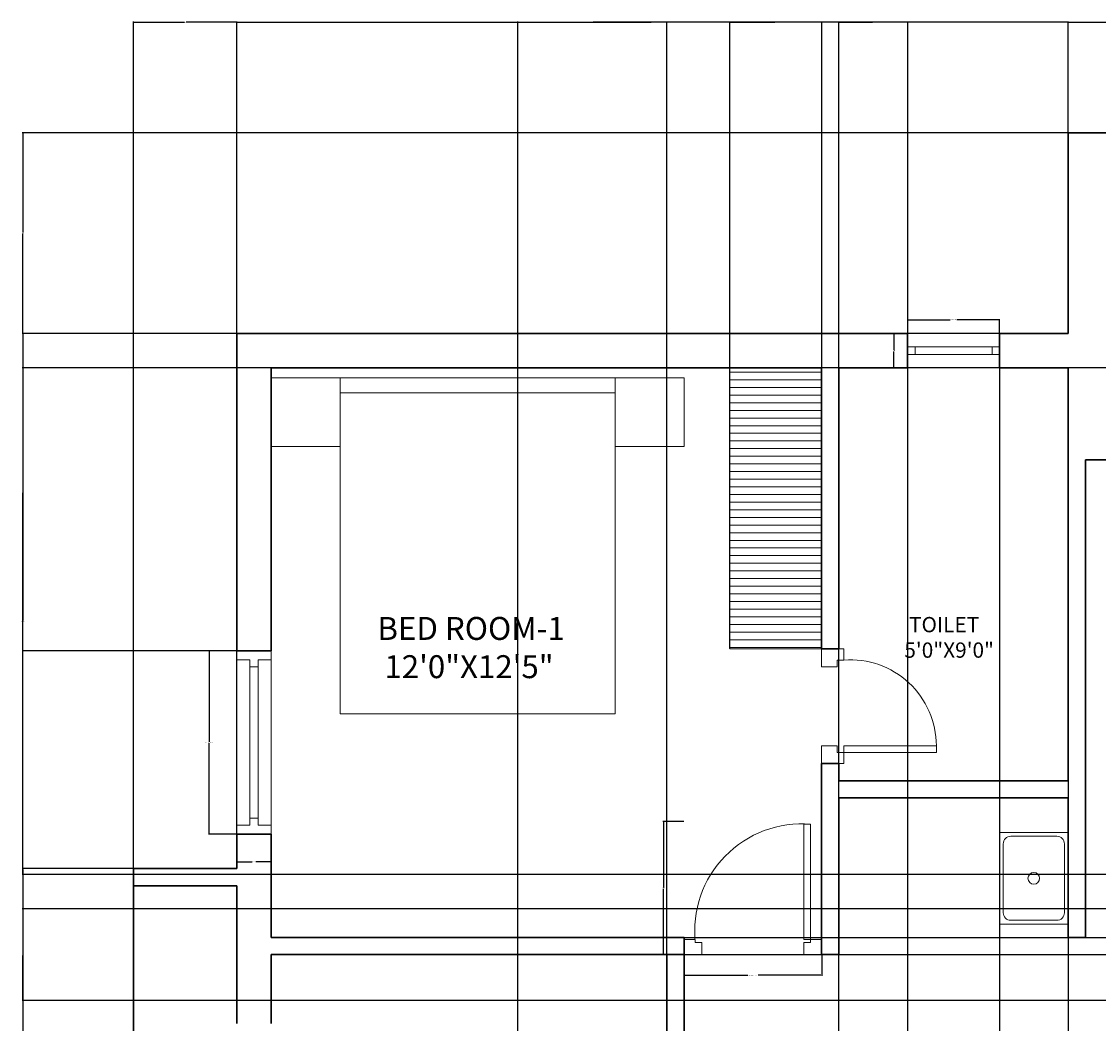
# Model space of a CAD drawing. Units: inches. Extents: x 2134 to 2768, y 715 to 1206.
# Tile 2 of 4: x 2134 to 2416, y 944 to 1206. Entities that reach past the tile are written whole.
import ezdxf

# ---------------------------------------------------------------- set-up
doc = ezdxf.new("R2010")
doc.units = ezdxf.units.IN
for name, color, linetype, lineweight in [('A-ANNO-DIMS', 2, 'Continuous', 18), ('A-AREA-IDEN', 7, 'Continuous', 18), ('A-DOOR', 251, 'Continuous', 13), ('A-FLOR-CASE', 251, 'Continuous', 13), ('A-FLOR-CASE-PATT', 252, 'Continuous', 9), ('A-FLOR-FIXT', 9, 'Continuous', 13), ('A-FURN', 251, 'Continuous', 13), ('A-WALL', 7, 'Continuous', 30), ('A-WINDOW', 251, 'Continuous', 13)]:
    doc.layers.add(name, color=color, linetype=linetype, lineweight=lineweight)
doc.styles.get("Standard").update_dxf_attribs({"font": 'arial.ttf'})
doc.dimstyles.get("Standard").update_dxf_attribs({"dimtxt": 0.18, "dimasz": 0.18, "dimexe": 0.18, "dimexo": 0.0625, "dimgap": 0.09, "dimtad": 0, "dimtih": 1, "dimtoh": 1, "dimdec": 4, "dimzin": 0, "dimdsep": 46, "dimtxsty": 'Standard', "dimcen": 0.09, "dimadec": 0, "dimazin": 0, "dimtfac": 1, "dimtdec": 4, "dimtofl": 0, "dimtmove": 0, "dimatfit": 3, "dimfxl": 1, "dimtolj": 1, "dimtzin": 0, "dimarcsym": 0})

# ---------------------------------------------------------------- blocks, each defined once
blk = doc.blocks.new('ARCHITRAVE')
at = {"layer": 'A-DOOR'}
for p, q in [((0, 0), (0, 4)), ((0, 3.99), (2.92, 3.99)), ((2.92, 3.99), (2.92, 3.17)), ((2.92, 3.17), (4.67, 3.17)), ((4.67, 3.17), (4.67, 0)), ((4.67, 0), (0, 0))]:
    blk.add_line(p, q, dxfattribs=at)
blk = doc.blocks.new('3 FEET DOOR')
at = {"layer": 'A-DOOR'}
blk.add_lwpolyline([(-34.02, 3.98), (-34.02, 34.15), (-32.27, 34.15), (-32.27, 3.98)], close=True, dxfattribs=at)
at = {"layer": 'A-DOOR', "ltscale": 0.1}
blk.add_arc((-31.74, 6.19), 28.05, 353.8214, 94.662, dxfattribs=at)
at = {"layer": 'A-DOOR'}
blk.add_blockref('ARCHITRAVE', (-36.91, 0), dxfattribs=at)
at = {"layer": 'A-DOOR', "xscale": -1}
blk.add_blockref('ARCHITRAVE', (-0.93, 0), dxfattribs=at)
blk = doc.blocks.new('2 feet 6 inch door')
at = {"layer": 'A-DOOR'}
for points in [[(2.92, 5.83), (2.92, 30), (4.67, 30), (4.67, 5.83)], [(2.92, 4.08), (4.67, 4.08), (4.67, 0), (0, 0), (0, 5.83), (2.92, 5.83)], [(27.08, 5.83), (27.08, 4.08), (25.33, 4.08), (25.33, 0), (30, 0), (30, 5.83)]]:
    blk.add_lwpolyline(points, close=True, dxfattribs=at)
at = {"layer": 'A-DOOR', "ltscale": 0.1}
blk.add_arc((4.67, 7.52), 22.48, 355.6972, 90, dxfattribs=at)
blk = doc.blocks.new('bed')
at = {"layer": 'A-FURN'}
for points in [[(3369.68, 925.24), (3297.68, 925.24), (3297.68, 1009.24), (3369.68, 1009.24)], [(3297.68, 921.32), (3279.68, 921.32), (3279.68, 939.32), (3297.68, 939.32)], [(3369.68, 921.32), (3387.68, 921.32), (3387.68, 939.32), (3369.68, 939.32)], [(3297.68, 925.24), (3369.68, 925.24), (3369.68, 921.32), (3297.68, 921.32)]]:
    blk.add_lwpolyline(points, close=True, dxfattribs=at)
blk = doc.blocks.new('WINDOW FRAME')
at = {"layer": 'A-WINDOW'}
for points in [[(4178.2, 4970.76), (4174.8, 4970.76), (4174.8, 4968.41), (4183.8, 4968.41), (4183.8, 4970.76), (4180.39, 4970.76)], [(4180.39, 4970.76), (4180.39, 4972.59), (4178.2, 4972.59), (4178.2, 4970.76)]]:
    blk.add_lwpolyline(points, dxfattribs=at)
blk = doc.blocks.new("4' window")
at = {"layer": 'A-WINDOW'}
for p, q in [((2.35, 9), (45.65, 9)), ((43.82, 5.59), (4.18, 5.59)), ((43.82, 3.41), (4.18, 3.41)), ((2.35, 0), (45.65, 0))]:
    blk.add_line(p, q, dxfattribs=at)
at = {"layer": 'A-WINDOW', "rotation": 270}
blk.add_blockref('WINDOW FRAME', (-4968.41, 4183.8), dxfattribs=at)
at = {"layer": 'A-WINDOW', "xscale": -1, "rotation": 90}
blk.add_blockref('WINDOW FRAME', (5016.41, 4183.8), dxfattribs=at)
blk = doc.blocks.new("2' ventilators")
at = {"layer": 'A-WINDOW'}
for p, q in [((24, 5.5), (0, 5.5)), ((1.93, 5.5), (1.93, 3.5)), ((22.07, 5.5), (22.07, 3.5))]:
    blk.add_line(p, q, dxfattribs=at)
for points in [[(0, 9), (24, 9), (24, 0), (0, 0), (0, 9)], [(24, 3.5), (0, 3.5)]]:
    blk.add_lwpolyline(points, dxfattribs=at)
blk = doc.blocks.new('sink')
at = {"layer": 'A-FURN'}
for p, q in [((-9, 12), (9, 12)), ((-9, -12), (-9, 12)), ((9, 12), (9, -12)), ((-8, -9), (-8, 9)), ((-6, 11), (6, 11)), ((8, 9), (8, -9)), ((6, -11), (-6, -11)), ((9, -12), (-9, -12))]:
    blk.add_line(p, q, dxfattribs=at)
blk.add_circle((0, 0), 1.53, dxfattribs=at)
for centre, start, end in [((-6, 9), 90, 180), ((6, 9), 0, 90), ((-6, -9), 180, 270), ((6, -9), 270, 0)]:
    blk.add_arc(centre, 2, start, end, dxfattribs=at)
blk = doc.blocks.new('*D51')
at = {"layer": 'A-ANNO-DIMS', "color": 0, "lineweight": -2, "transparency": 16777216}
for p, q in [((2307.81, 961.54), (2307.81, 956.03)), ((2343.79, 961.54), (2343.79, 956.03)), ((2307.99, 956.21), (2324.44, 956.21)), ((2343.61, 956.21), (2327.16, 956.21))]:
    blk.add_line(p, q, dxfattribs=at)
at = {"layer": 'A-ANNO-DIMS', "color": 0, "transparency": 16777216}
for points in [[(2307.99, 956.24), (2307.99, 956.18), (2307.81, 956.21)], [(2343.61, 956.24), (2343.61, 956.18), (2343.79, 956.21)]]:
    blk.add_solid(points, dxfattribs=at)
at = {"layer": 'Defpoints', "color": 0, "transparency": 16777216}
for p in [(2307.81, 961.61), (2343.79, 961.61), (2307.81, 956.21)]:
    blk.add_point(p, dxfattribs=at)
at = {"layer": 'A-ANNO-DIMS', "color": 0, "transparency": 16777216, "insert": (2325.8, 956.21), "char_height": 0.18, "attachment_point": 5}
blk.add_mtext('\\A1;ROOM DOOR 36 TYP.', dxfattribs=at)
blk = doc.blocks.new('*D52')
at = {"layer": 'A-ANNO-DIMS', "color": 0, "lineweight": -2, "transparency": 16777216}
for p, q in [((2307.75, 996.43), (2302.24, 996.43)), ((2302.42, 996.25), (2302.42, 979.2)), ((2302.42, 961.79), (2302.42, 978.84)), ((2307.75, 961.61), (2302.24, 961.61))]:
    blk.add_line(p, q, dxfattribs=at)
at = {"layer": 'A-ANNO-DIMS', "color": 0, "transparency": 16777216}
for points in [[(2302.39, 996.25), (2302.45, 996.25), (2302.42, 996.43)], [(2302.39, 961.79), (2302.45, 961.79), (2302.42, 961.61)]]:
    blk.add_solid(points, dxfattribs=at)
at = {"layer": 'Defpoints', "color": 0, "transparency": 16777216}
for p in [(2302.42, 996.43), (2307.81, 996.43), (2307.81, 961.61)]:
    blk.add_point(p, dxfattribs=at)
at = {"layer": 'A-ANNO-DIMS', "color": 0, "transparency": 16777216, "insert": (2302.42, 979.02), "char_height": 0.18, "attachment_point": 5}
blk.add_mtext('\\A1;35 TYP.', dxfattribs=at)
blk = doc.blocks.new('*D57')
at = {"layer": 'A-ANNO-DIMS', "color": 0, "lineweight": -2, "transparency": 16777216}
for p, q in [((2366.29, 1124.17), (2366.29, 1127.89)), ((2366.47, 1127.71), (2377.38, 1127.71)), ((2390.11, 1127.71), (2379.19, 1127.71)), ((2390.29, 1124.17), (2390.29, 1127.89))]:
    blk.add_line(p, q, dxfattribs=at)
at = {"layer": 'A-ANNO-DIMS', "color": 0, "transparency": 16777216}
for points in [[(2366.47, 1127.74), (2366.47, 1127.68), (2366.29, 1127.71)], [(2390.11, 1127.74), (2390.11, 1127.68), (2390.29, 1127.71)]]:
    blk.add_solid(points, dxfattribs=at)
at = {"layer": 'Defpoints', "color": 0, "transparency": 16777216}
for p in [(2390.29, 1127.71), (2366.29, 1124.11), (2390.29, 1124.11)]:
    blk.add_point(p, dxfattribs=at)
at = {"layer": 'A-ANNO-DIMS', "color": 0, "transparency": 16777216, "insert": (2378.29, 1127.71), "char_height": 0.18, "attachment_point": 5}
blk.add_mtext('\\A1;VENT 24 TYP.', dxfattribs=at)
blk = doc.blocks.new('*D58')
at = {"layer": 'A-ANNO-DIMS', "color": 0, "lineweight": -2, "transparency": 16777216}
for p, q in [((2366.22, 1124.11), (2362.51, 1124.11)), ((2362.69, 1123.93), (2362.69, 1119.79)), ((2362.69, 1115.29), (2362.69, 1119.43)), ((2366.22, 1115.11), (2362.51, 1115.11))]:
    blk.add_line(p, q, dxfattribs=at)
at = {"layer": 'A-ANNO-DIMS', "color": 0, "transparency": 16777216}
for points in [[(2362.66, 1123.93), (2362.72, 1123.93), (2362.69, 1124.11)], [(2362.66, 1115.29), (2362.72, 1115.29), (2362.69, 1115.11)]]:
    blk.add_solid(points, dxfattribs=at)
at = {"layer": 'Defpoints', "color": 0, "transparency": 16777216}
for p in [(2362.69, 1124.11), (2366.29, 1124.11), (2366.29, 1115.11)]:
    blk.add_point(p, dxfattribs=at)
at = {"layer": 'A-ANNO-DIMS', "color": 0, "transparency": 16777216, "insert": (2362.69, 1119.61), "char_height": 0.18, "attachment_point": 5}
blk.add_mtext('\\A1;9 TYP.', dxfattribs=at)
blk = doc.blocks.new('*D59')
at = {"layer": 'A-ANNO-DIMS', "color": 0, "lineweight": -2, "transparency": 16777216}
for p, q in [((2190.72, 1041.11), (2183.41, 1041.11)), ((2183.59, 1040.93), (2183.59, 1017.29)), ((2183.59, 993.29), (2183.59, 1016.92)), ((2190.72, 993.11), (2183.41, 993.11))]:
    blk.add_line(p, q, dxfattribs=at)
at = {"layer": 'A-ANNO-DIMS', "color": 0, "transparency": 16777216}
for points in [[(2183.56, 1040.93), (2183.62, 1040.93), (2183.59, 1041.11)], [(2183.56, 993.29), (2183.62, 993.29), (2183.59, 993.11)]]:
    blk.add_solid(points, dxfattribs=at)
at = {"layer": 'Defpoints', "color": 0, "transparency": 16777216}
for p in [(2190.79, 1041.11), (2183.59, 993.11), (2190.79, 993.11)]:
    blk.add_point(p, dxfattribs=at)
at = {"layer": 'A-ANNO-DIMS', "color": 0, "transparency": 16777216, "insert": (2183.59, 1017.11), "char_height": 0.18, "attachment_point": 5}
blk.add_mtext('\\A1;WINDOW 48 TYP.', dxfattribs=at)
blk = doc.blocks.new('*D60')
at = {"layer": 'A-ANNO-DIMS', "color": 0, "lineweight": -2, "transparency": 16777216}
for p, q in [((2190.79, 993.04), (2190.79, 985.73)), ((2199.79, 993.04), (2199.79, 985.73)), ((2190.97, 985.91), (2194.83, 985.91)), ((2199.61, 985.91), (2195.75, 985.91))]:
    blk.add_line(p, q, dxfattribs=at)
at = {"layer": 'A-ANNO-DIMS', "color": 0, "transparency": 16777216}
for points in [[(2190.97, 985.94), (2190.97, 985.88), (2190.79, 985.91)], [(2199.61, 985.94), (2199.61, 985.88), (2199.79, 985.91)]]:
    blk.add_solid(points, dxfattribs=at)
at = {"layer": 'Defpoints', "color": 0, "transparency": 16777216}
for p in [(2190.79, 993.11), (2199.79, 993.11), (2199.79, 985.91)]:
    blk.add_point(p, dxfattribs=at)
at = {"layer": 'A-ANNO-DIMS', "color": 0, "transparency": 16777216, "insert": (2195.29, 985.91), "char_height": 0.18, "attachment_point": 5}
blk.add_mtext('\\A1;9 TYP.', dxfattribs=at)
blk = doc.blocks.new('*D77')
at = {"layer": 'A-ANNO-DIMS', "color": 0, "lineweight": -2, "transparency": 16777216}
for p, q in [((2190.79, 1124.17), (2190.79, 1205.74)), ((2190.97, 1205.56), (2299.14, 1205.56)), ((2408.11, 1205.56), (2299.93, 1205.56)), ((2408.29, 1124.17), (2408.29, 1205.74))]:
    blk.add_line(p, q, dxfattribs=at)
at = {"layer": 'A-ANNO-DIMS', "color": 0, "transparency": 16777216}
for points in [[(2190.97, 1205.59), (2190.97, 1205.53), (2190.79, 1205.56)], [(2408.11, 1205.59), (2408.11, 1205.53), (2408.29, 1205.56)]]:
    blk.add_solid(points, dxfattribs=at)
at = {"layer": 'Defpoints', "color": 0, "transparency": 16777216}
for p in [(2408.29, 1205.56), (2190.79, 1124.11), (2408.29, 1124.11)]:
    blk.add_point(p, dxfattribs=at)
at = {"layer": 'A-ANNO-DIMS', "color": 0, "transparency": 16777216, "insert": (2299.54, 1205.56), "char_height": 0.18, "attachment_point": 5}
blk.add_mtext('\\A1;217.5', dxfattribs=at)
blk = doc.blocks.new('*D78')
at = {"layer": 'A-ANNO-DIMS', "color": 0, "lineweight": -2, "transparency": 16777216}
for p, q in [((2408.29, 1176.67), (2408.29, 1205.74)), ((2408.47, 1205.56), (2478.65, 1205.56)), ((2549.61, 1205.56), (2479.42, 1205.56)), ((2549.79, 1176.67), (2549.79, 1205.74))]:
    blk.add_line(p, q, dxfattribs=at)
at = {"layer": 'A-ANNO-DIMS', "color": 0, "transparency": 16777216}
for points in [[(2408.47, 1205.59), (2408.47, 1205.53), (2408.29, 1205.56)], [(2549.61, 1205.59), (2549.61, 1205.53), (2549.79, 1205.56)]]:
    blk.add_solid(points, dxfattribs=at)
at = {"layer": 'Defpoints', "color": 0, "transparency": 16777216}
for p in [(2549.79, 1205.56), (2408.29, 1176.61), (2549.79, 1176.61)]:
    blk.add_point(p, dxfattribs=at)
at = {"layer": 'A-ANNO-DIMS', "color": 0, "transparency": 16777216, "insert": (2479.04, 1205.56), "char_height": 0.18, "attachment_point": 5}
blk.add_mtext('\\A1;141.5', dxfattribs=at)
blk = doc.blocks.new('*D79')
at = {"layer": 'A-ANNO-DIMS', "color": 0, "lineweight": -2, "transparency": 16777216}
for p, q in [((2408.22, 1176.61), (2134.66, 1176.61)), ((2134.84, 1176.43), (2134.84, 1150.54)), ((2134.84, 1124.29), (2134.84, 1150.18)), ((2408.22, 1124.11), (2134.66, 1124.11))]:
    blk.add_line(p, q, dxfattribs=at)
at = {"layer": 'A-ANNO-DIMS', "color": 0, "transparency": 16777216}
for points in [[(2134.81, 1176.43), (2134.87, 1176.43), (2134.84, 1176.61)], [(2134.81, 1124.29), (2134.87, 1124.29), (2134.84, 1124.11)]]:
    blk.add_solid(points, dxfattribs=at)
at = {"layer": 'Defpoints', "color": 0, "transparency": 16777216}
for p in [(2134.84, 1176.61), (2408.29, 1176.61), (2408.29, 1124.11)]:
    blk.add_point(p, dxfattribs=at)
at = {"layer": 'A-ANNO-DIMS', "color": 0, "transparency": 16777216, "insert": (2134.84, 1150.36), "char_height": 0.18, "attachment_point": 5}
blk.add_mtext('\\A1;52.5', dxfattribs=at)
blk = doc.blocks.new('*D80')
at = {"layer": 'A-ANNO-DIMS', "color": 0, "lineweight": -2, "transparency": 16777216}
for p, q in [((2163.79, 984.17), (2163.79, 1205.74)), ((2163.97, 1205.56), (2177.07, 1205.56)), ((2190.61, 1205.56), (2177.51, 1205.56)), ((2190.79, 984.17), (2190.79, 1205.74))]:
    blk.add_line(p, q, dxfattribs=at)
at = {"layer": 'A-ANNO-DIMS', "color": 0, "transparency": 16777216}
for points in [[(2163.97, 1205.59), (2163.97, 1205.53), (2163.79, 1205.56)], [(2190.61, 1205.59), (2190.61, 1205.53), (2190.79, 1205.56)]]:
    blk.add_solid(points, dxfattribs=at)
at = {"layer": 'Defpoints', "color": 0, "transparency": 16777216}
for p in [(2190.79, 1205.56), (2163.79, 984.11), (2190.79, 984.11)]:
    blk.add_point(p, dxfattribs=at)
at = {"layer": 'A-ANNO-DIMS', "color": 0, "transparency": 16777216, "insert": (2177.29, 1205.56), "char_height": 0.18, "attachment_point": 5}
blk.add_mtext('\\A1;27', dxfattribs=at)
blk = doc.blocks.new('*D82')
at = {"layer": 'A-ANNO-DIMS', "color": 0, "lineweight": -2, "transparency": 16777216}
for p, q in [((2163.72, 984.11), (2134.66, 984.11)), ((2134.84, 983.93), (2134.84, 940.79)), ((2134.84, 897.29), (2134.84, 940.43)), ((2163.72, 897.11), (2134.66, 897.11))]:
    blk.add_line(p, q, dxfattribs=at)
at = {"layer": 'A-ANNO-DIMS', "color": 0, "transparency": 16777216}
for points in [[(2134.81, 983.93), (2134.87, 983.93), (2134.84, 984.11)], [(2134.81, 897.29), (2134.87, 897.29), (2134.84, 897.11)]]:
    blk.add_solid(points, dxfattribs=at)
at = {"layer": 'Defpoints', "color": 0, "transparency": 16777216}
for p in [(2134.84, 984.11), (2163.79, 984.11), (2163.79, 897.11)]:
    blk.add_point(p, dxfattribs=at)
at = {"layer": 'A-ANNO-DIMS', "color": 0, "transparency": 16777216, "insert": (2134.84, 940.61), "char_height": 0.18, "attachment_point": 5}
blk.add_mtext('\\A1;87', dxfattribs=at)
blk = doc.blocks.new('*D83')
at = {"layer": 'A-ANNO-DIMS', "color": 0, "lineweight": -2, "transparency": 16777216}
for p, q in [((2348.29, 753.17), (2348.29, 1205.74)), ((2348.47, 1205.56), (2357.08, 1205.56)), ((2366.11, 1205.56), (2357.5, 1205.56)), ((2366.29, 753.17), (2366.29, 1205.74))]:
    blk.add_line(p, q, dxfattribs=at)
at = {"layer": 'A-ANNO-DIMS', "color": 0, "transparency": 16777216}
for points in [[(2348.47, 1205.59), (2348.47, 1205.53), (2348.29, 1205.56)], [(2366.11, 1205.59), (2366.11, 1205.53), (2366.29, 1205.56)]]:
    blk.add_solid(points, dxfattribs=at)
at = {"layer": 'Defpoints', "color": 0, "transparency": 16777216}
for p in [(2366.29, 1205.56), (2348.29, 753.11), (2366.29, 753.11)]:
    blk.add_point(p, dxfattribs=at)
at = {"layer": 'A-ANNO-DIMS', "color": 0, "transparency": 16777216, "insert": (2357.29, 1205.56), "char_height": 0.18, "attachment_point": 5}
blk.add_mtext('\\A1;18', dxfattribs=at)
blk = doc.blocks.new('*D87')
at = {"layer": 'A-ANNO-DIMS', "color": 0, "lineweight": -2, "transparency": 16777216}
for p, q in [((2190.72, 1124.11), (2134.66, 1124.11)), ((2134.84, 1123.93), (2134.84, 1082.79)), ((2134.84, 1041.29), (2134.84, 1082.43)), ((2190.72, 1041.11), (2134.66, 1041.11))]:
    blk.add_line(p, q, dxfattribs=at)
at = {"layer": 'A-ANNO-DIMS', "color": 0, "transparency": 16777216}
for points in [[(2134.81, 1123.93), (2134.87, 1123.93), (2134.84, 1124.11)], [(2134.81, 1041.29), (2134.87, 1041.29), (2134.84, 1041.11)]]:
    blk.add_solid(points, dxfattribs=at)
at = {"layer": 'Defpoints', "color": 0, "transparency": 16777216}
for p in [(2190.79, 1124.11), (2134.84, 1041.11), (2190.79, 1041.11)]:
    blk.add_point(p, dxfattribs=at)
at = {"layer": 'A-ANNO-DIMS', "color": 0, "transparency": 16777216, "insert": (2134.84, 1082.61), "char_height": 0.18, "attachment_point": 5}
blk.add_mtext('\\A1;83', dxfattribs=at)
blk = doc.blocks.new('*D89')
at = {"layer": 'A-ANNO-DIMS', "color": 0, "lineweight": -2, "transparency": 16777216}
for p, q in [((2729.72, 973.61), (2134.66, 973.61)), ((2134.84, 973.43), (2134.84, 961.79)), ((2134.84, 949.79), (2134.84, 961.43)), ((2729.72, 949.61), (2134.66, 949.61))]:
    blk.add_line(p, q, dxfattribs=at)
at = {"layer": 'A-ANNO-DIMS', "color": 0, "transparency": 16777216}
for points in [[(2134.81, 973.43), (2134.87, 973.43), (2134.84, 973.61)], [(2134.81, 949.79), (2134.87, 949.79), (2134.84, 949.61)]]:
    blk.add_solid(points, dxfattribs=at)
at = {"layer": 'Defpoints', "color": 0, "transparency": 16777216}
for p in [(2134.84, 973.61), (2729.79, 973.61), (2729.79, 949.61)]:
    blk.add_point(p, dxfattribs=at)
at = {"layer": 'A-ANNO-DIMS', "color": 0, "transparency": 16777216, "insert": (2134.84, 961.61), "char_height": 0.18, "attachment_point": 5}
blk.add_mtext('\\A1;24', dxfattribs=at)
blk = doc.blocks.new('*D91')
at = {"layer": 'A-ANNO-DIMS', "color": 0, "lineweight": -2, "transparency": 16777216}
for p, q in [((2390.29, 1115.04), (2390.29, 714.98)), ((2408.29, 1115.04), (2408.29, 714.98)), ((2390.47, 715.16), (2399.08, 715.16)), ((2408.11, 715.16), (2399.5, 715.16))]:
    blk.add_line(p, q, dxfattribs=at)
at = {"layer": 'A-ANNO-DIMS', "color": 0, "transparency": 16777216}
for points in [[(2390.47, 715.19), (2390.47, 715.13), (2390.29, 715.16)], [(2408.11, 715.19), (2408.11, 715.13), (2408.29, 715.16)]]:
    blk.add_solid(points, dxfattribs=at)
at = {"layer": 'Defpoints', "color": 0, "transparency": 16777216}
for p in [(2390.29, 1115.11), (2408.29, 1115.11), (2408.29, 715.16)]:
    blk.add_point(p, dxfattribs=at)
at = {"layer": 'A-ANNO-DIMS', "color": 0, "transparency": 16777216, "insert": (2399.29, 715.16), "char_height": 0.18, "attachment_point": 5}
blk.add_mtext('\\A1;18', dxfattribs=at)
blk = doc.blocks.new('*D95')
at = {"layer": 'A-ANNO-DIMS', "color": 0, "lineweight": -2, "transparency": 16777216}
for p, q in [((2549.72, 973.61), (2134.66, 973.61)), ((2134.84, 973.43), (2134.84, 961.79)), ((2134.84, 949.79), (2134.84, 961.43)), ((2549.72, 949.61), (2134.66, 949.61))]:
    blk.add_line(p, q, dxfattribs=at)
at = {"layer": 'A-ANNO-DIMS', "color": 0, "transparency": 16777216}
for points in [[(2134.81, 973.43), (2134.87, 973.43), (2134.84, 973.61)], [(2134.81, 949.79), (2134.87, 949.79), (2134.84, 949.61)]]:
    blk.add_solid(points, dxfattribs=at)
at = {"layer": 'Defpoints', "color": 0, "transparency": 16777216}
for p in [(2549.79, 973.61), (2134.84, 949.61), (2549.79, 949.61)]:
    blk.add_point(p, dxfattribs=at)
at = {"layer": 'A-ANNO-DIMS', "color": 0, "transparency": 16777216, "insert": (2134.84, 961.61), "char_height": 0.18, "attachment_point": 5}
blk.add_mtext('\\A1;24', dxfattribs=at)
blk = doc.blocks.new('*D100')
at = {"layer": 'A-ANNO-DIMS', "color": 0, "lineweight": -2, "transparency": 16777216}
for p, q in [((2679.72, 1115.11), (2134.66, 1115.11)), ((2134.84, 1114.93), (2134.84, 1049.03)), ((2134.84, 982.77), (2134.84, 1048.67)), ((2679.72, 982.59), (2134.66, 982.59))]:
    blk.add_line(p, q, dxfattribs=at)
at = {"layer": 'A-ANNO-DIMS', "color": 0, "transparency": 16777216}
for points in [[(2134.81, 1114.93), (2134.87, 1114.93), (2134.84, 1115.11)], [(2134.81, 982.77), (2134.87, 982.77), (2134.84, 982.59)]]:
    blk.add_solid(points, dxfattribs=at)
at = {"layer": 'Defpoints', "color": 0, "transparency": 16777216}
for p in [(2679.79, 1115.11), (2134.84, 982.59), (2679.79, 982.59)]:
    blk.add_point(p, dxfattribs=at)
at = {"layer": 'A-ANNO-DIMS', "color": 0, "transparency": 16777216, "insert": (2134.84, 1048.85), "char_height": 0.18, "attachment_point": 5}
blk.add_mtext('\\A1;132.52', dxfattribs=at)
blk = doc.blocks.new('*D101')
at = {"layer": 'A-ANNO-DIMS', "color": 0, "lineweight": -2, "transparency": 16777216}
for p, q in [((2319.79, 1041.67), (2319.79, 1205.74)), ((2319.97, 1205.56), (2331.57, 1205.56)), ((2343.61, 1205.56), (2332.01, 1205.56)), ((2343.79, 1041.67), (2343.79, 1205.74))]:
    blk.add_line(p, q, dxfattribs=at)
at = {"layer": 'A-ANNO-DIMS', "color": 0, "transparency": 16777216}
for points in [[(2319.97, 1205.59), (2319.97, 1205.53), (2319.79, 1205.56)], [(2343.61, 1205.59), (2343.61, 1205.53), (2343.79, 1205.56)]]:
    blk.add_solid(points, dxfattribs=at)
at = {"layer": 'Defpoints', "color": 0, "transparency": 16777216}
for p in [(2343.79, 1205.56), (2319.79, 1041.61), (2343.79, 1041.61)]:
    blk.add_point(p, dxfattribs=at)
at = {"layer": 'A-ANNO-DIMS', "color": 0, "transparency": 16777216, "insert": (2331.79, 1205.56), "char_height": 0.18, "attachment_point": 5}
blk.add_mtext('\\A1;24', dxfattribs=at)
blk = doc.blocks.new('*D102')
at = {"layer": 'A-ANNO-DIMS', "color": 0, "lineweight": -2, "transparency": 16777216}
for p, q in [((2199.85, 966.11), (2767.92, 966.11)), ((2767.74, 965.93), (2767.74, 964.04)), ((2767.74, 961.79), (2767.74, 963.68)), ((2199.85, 961.61), (2767.92, 961.61))]:
    blk.add_line(p, q, dxfattribs=at)
at = {"layer": 'A-ANNO-DIMS', "color": 0, "transparency": 16777216}
for points in [[(2767.71, 965.93), (2767.77, 965.93), (2767.74, 966.11)], [(2767.71, 961.79), (2767.77, 961.79), (2767.74, 961.61)]]:
    blk.add_solid(points, dxfattribs=at)
at = {"layer": 'Defpoints', "color": 0, "transparency": 16777216}
for p in [(2199.79, 966.11), (2767.74, 966.11), (2199.79, 961.61)]:
    blk.add_point(p, dxfattribs=at)
at = {"layer": 'A-ANNO-DIMS', "color": 0, "transparency": 16777216, "insert": (2767.74, 963.86), "char_height": 0.18, "attachment_point": 5}
blk.add_mtext('\\A1;4.5', dxfattribs=at)
blk = doc.blocks.new('*D103')
at = {"layer": 'A-ANNO-DIMS', "color": 0, "lineweight": -2, "transparency": 16777216}
for p, q in [((2264.29, 901.67), (2264.29, 1205.74)), ((2264.47, 1205.56), (2283.57, 1205.56)), ((2303.11, 1205.56), (2284.01, 1205.56)), ((2303.29, 901.67), (2303.29, 1205.74))]:
    blk.add_line(p, q, dxfattribs=at)
at = {"layer": 'A-ANNO-DIMS', "color": 0, "transparency": 16777216}
for points in [[(2264.47, 1205.59), (2264.47, 1205.53), (2264.29, 1205.56)], [(2303.11, 1205.59), (2303.11, 1205.53), (2303.29, 1205.56)]]:
    blk.add_solid(points, dxfattribs=at)
at = {"layer": 'Defpoints', "color": 0, "transparency": 16777216}
for p in [(2303.29, 1205.56), (2264.29, 901.61), (2303.29, 901.61)]:
    blk.add_point(p, dxfattribs=at)
at = {"layer": 'A-ANNO-DIMS', "color": 0, "transparency": 16777216, "insert": (2283.79, 1205.56), "char_height": 0.18, "attachment_point": 5}
blk.add_mtext('\\A1;39', dxfattribs=at)

msp = doc.modelspace()

# ---------------------------------------------------------------- hatches: boundary and pattern name
at = {"layer": 'A-FLOR-CASE-PATT'}
h = msp.add_hatch(dxfattribs=at)
h.set_pattern_fill('_USER', color=256, scale=2, pattern_type=0)
h.set_pattern_definition([(0, (0, 0), (0, 2), [])])
h.paths.add_polyline_path([(2343.787, 1115.107), (2319.787, 1115.107), (2319.787, 1041.607), (2343.787, 1041.607)])

# ---------------------------------------------------------------- linework, layer by layer
at = {"layer": 'A-FLOR-CASE'}
for p, q in [((2319.787, 1115.107), (2319.787, 1041.607)), ((2319.787, 1041.607), (2343.787, 1041.607)), ((2390.287, 1002.607), (2390.287, 966.107)), ((2390.287, 966.107), (2408.287, 966.107))]:
    msp.add_line(p, q, dxfattribs=at)
at = {"layer": 'A-WALL'}
for p, q in [((2408.287, 1176.607), (2408.287, 1124.107)), ((2408.287, 1176.607), (2549.787, 1176.607)), ((2190.787, 1124.107), (2190.787, 1041.107)), ((2366.287, 1124.107), (2190.787, 1124.107)), ((2366.287, 1115.107), (2366.287, 1124.107)), ((2408.287, 1124.107), (2390.287, 1124.107)), ((2390.287, 1115.107), (2390.287, 1124.107)), ((2199.787, 1115.107), (2199.787, 1041.107)), ((2343.787, 1115.107), (2199.787, 1115.107)), ((2343.787, 1115.107), (2343.787, 1041.607)), ((2348.287, 1115.107), (2348.287, 1041.607)), ((2366.287, 1115.107), (2348.287, 1115.107)), ((2408.287, 1115.107), (2390.287, 1115.107)), ((2408.287, 1115.107), (2408.287, 1007.107)), ((2412.787, 1091.107), (2412.787, 966.107)), ((2443.037, 1091.107), (2412.787, 1091.107)), ((2190.787, 1041.107), (2199.787, 1041.107)), ((2348.287, 1041.607), (2343.787, 1041.607)), ((2348.287, 1011.607), (2343.787, 1011.607)), ((2343.787, 1011.607), (2343.787, 961.607)), ((2348.287, 1011.607), (2348.287, 1007.107)), ((2408.287, 1007.107), (2348.287, 1007.107)), ((2408.287, 1002.607), (2348.287, 1002.607)), ((2348.287, 1002.607), (2348.287, 961.607)), ((2408.287, 1002.607), (2408.287, 966.107)), ((2190.787, 993.107), (2199.787, 993.107)), ((2190.787, 993.107), (2190.787, 984.107)), ((2199.787, 993.107), (2199.787, 966.107)), ((2190.787, 984.107), (2163.787, 984.107)), ((2163.787, 979.607), (2163.787, 984.107)), ((2190.787, 979.607), (2163.787, 979.607)), ((2163.787, 979.607), (2163.787, 901.607)), ((2190.787, 979.607), (2190.787, 943.607)), ((2307.787, 966.107), (2199.787, 966.107)), ((2307.787, 966.107), (2307.787, 897.107)), ((2408.287, 966.107), (2412.787, 966.107)), ((2408.287, 966.107), (2412.787, 966.107)), ((2303.287, 961.607), (2199.787, 961.607)), ((2199.787, 961.607), (2199.787, 943.607)), ((2303.287, 961.607), (2303.287, 901.607)), ((2343.787, 961.607), (2348.287, 961.607))]:
    msp.add_line(p, q, dxfattribs=at)

# ---------------------------------------------------------------- block references
at = {"layer": 'A-DOOR', "xscale": -1, "rotation": 270}
msp.add_blockref('2 feet 6 inch door', (2343.787, 1011.607), dxfattribs=at)
at = {"layer": 'A-DOOR', "xscale": -1}
msp.add_blockref('3 FEET DOOR', (2306.88, 961.607), dxfattribs=at)
at = {"layer": 'A-FLOR-FIXT'}
msp.add_blockref('sink', (2399.287, 981.589), dxfattribs=at)
at = {"layer": 'A-FURN', "rotation": 180}
msp.add_blockref('bed', (5587.47, 2033.866), dxfattribs=at)
at = {"layer": 'A-WINDOW'}
msp.add_blockref("2' ventilators", (2366.287, 1115.107), dxfattribs=at)
at = {"layer": 'A-WINDOW', "rotation": 270}
msp.add_blockref("4' window", (2190.787, 1041.107), dxfattribs=at)

# ---------------------------------------------------------------- texts
at = {"layer": 'A-AREA-IDEN', "attachment_point": 1}
for s, insert, char_height in [('BED ROOM-1\\P 12\'0"X12\'5"', (2227.563, 1049.954), 6), ('  TOILET\\P 5\'0"X9\'0"', (2364.192, 1049.954), 4)]:
    msp.add_mtext_dynamic_manual_height_columns(s, width=55.72169, gutter_width=12.5, heights=[0], dxfattribs=dict(at, insert=insert, char_height=char_height))

# ---------------------------------------------------------------- dimensions: what is measured, and where the dimension line sits
at = {"layer": 'A-ANNO-DIMS'}
for base, p1, p2, override, picture, middle in [((2190.787, 1205.557), (2163.787, 984.107), (2190.787, 984.107), {"dimdec": 0, "dimlfac": 1, "dimrnd": 0, "dimzin": 0, "dimdsep": 46, "dimlunit": 2}, '*D80', (2177.287, 1205.557)), ((2408.287, 1205.557), (2190.787, 1124.107), (2408.287, 1124.107), {"dimdec": 1, "dimlfac": 1, "dimrnd": 0, "dimzin": 0, "dimdsep": 46, "dimlunit": 2}, '*D77', (2299.537, 1205.557)), ((2303.287, 1205.557), (2264.287, 901.607), (2303.287, 901.607), {"dimdec": 0, "dimlfac": 1, "dimrnd": 0, "dimzin": 0, "dimdsep": 46, "dimlunit": 2}, '*D103', (2283.787, 1205.557)), ((2343.787, 1205.557), (2319.787, 1041.607), (2343.787, 1041.607), {"dimdec": 0, "dimlfac": 1, "dimrnd": 0, "dimzin": 0, "dimdsep": 46, "dimlunit": 2}, '*D101', (2331.787, 1205.557)), ((2366.287, 1205.557), (2348.287, 753.107), (2366.287, 753.107), {"dimdec": 0, "dimlfac": 1, "dimrnd": 0, "dimzin": 0, "dimdsep": 46, "dimlunit": 2}, '*D83', (2357.287, 1205.557)), ((2549.787, 1205.557), (2408.287, 1176.607), (2549.787, 1176.607), {"dimdec": 1, "dimlfac": 1, "dimrnd": 0, "dimzin": 0, "dimdsep": 46, "dimlunit": 2}, '*D78', (2479.037, 1205.557)), ((2408.287, 715.157), (2390.287, 1115.107), (2408.287, 1115.107), {"dimdec": 0, "dimlfac": 1, "dimrnd": 0, "dimzin": 0, "dimdsep": 46, "dimlunit": 2}, '*D91', (2399.287, 715.157))]:
    dim = msp.add_linear_dim(base=base, p1=p1, p2=p2, dimstyle='Standard', override=override, dxfattribs=at)
    dim.commit()
    dim.dimension.update_dxf_attribs({"geometry": picture, "text_midpoint": middle})
for base, p1, p2, override, picture, middle in [((2134.837, 1176.607), (2408.287, 1124.107), (2408.287, 1176.607), {"dimdec": 1, "dimlfac": 1, "dimrnd": 0, "dimzin": 0, "dimdsep": 46, "dimlunit": 2}, '*D79', (2134.837, 1150.357)), ((2134.837, 1041.107), (2190.787, 1124.107), (2190.787, 1041.107), {"dimdec": 0, "dimlfac": 1, "dimrnd": 0, "dimzin": 0, "dimdsep": 46, "dimlunit": 2}, '*D87', (2134.837, 1082.607)), ((2134.837, 982.591), (2679.787, 1115.107), (2679.787, 982.591), {"dimdec": 2, "dimlfac": 1, "dimrnd": 0, "dimzin": 0, "dimdsep": 46, "dimlunit": 2}, '*D100', (2134.837, 1048.849)), ((2134.837, 984.107), (2163.787, 897.107), (2163.787, 984.107), {"dimdec": 0, "dimlfac": 1, "dimrnd": 0, "dimzin": 0, "dimdsep": 46, "dimlunit": 2}, '*D82', (2134.837, 940.607)), ((2134.837, 973.607), (2729.787, 949.607), (2729.787, 973.607), {"dimdec": 0, "dimlfac": 1, "dimrnd": 0, "dimzin": 0, "dimdsep": 46, "dimlunit": 2}, '*D89', (2134.837, 961.607)), ((2134.837, 949.607), (2549.787, 973.607), (2549.787, 949.607), {"dimdec": 0, "dimlfac": 1, "dimrnd": 0, "dimzin": 0, "dimdsep": 46, "dimlunit": 2}, '*D95', (2134.837, 961.607)), ((2767.737, 966.107), (2199.787, 961.607), (2199.787, 966.107), {"dimdec": 1, "dimlfac": 1, "dimrnd": 0, "dimzin": 0, "dimdsep": 46, "dimlunit": 2}, '*D102', (2767.737, 963.857))]:
    dim = msp.add_linear_dim(base=base, p1=p1, p2=p2, angle=90, dimstyle='Standard', override=override, dxfattribs=at)
    dim.commit()
    dim.dimension.update_dxf_attribs({"geometry": picture, "text_midpoint": middle})
for base, p1, p2, text, picture, middle in [((2390.287, 1127.707), (2366.287, 1124.107), (2390.287, 1124.107), 'VENT <> TYP.', '*D57', (2378.287, 1127.707)), ((2199.787, 985.907), (2190.787, 993.107), (2199.787, 993.107), '<> TYP.', '*D60', (2195.287, 985.907))]:
    dim = msp.add_linear_dim(base=base, p1=p1, p2=p2, text=text, dimstyle='Standard', override={"dimdec": 0, "dimlfac": 1, "dimrnd": 0, "dimzin": 0, "dimdsep": 46, "dimlunit": 2}, dxfattribs=at)
    dim.commit()
    dim.dimension.update_dxf_attribs({"geometry": picture, "text_midpoint": middle})
for base, p1, p2, angle, text, picture, middle in [((2362.687, 1124.107), (2366.287, 1115.107), (2366.287, 1124.107), 90, '<> TYP.', '*D58', (2362.687, 1119.607)), ((2183.587, 993.107), (2190.787, 1041.107), (2190.787, 993.107), 270, 'WINDOW <> TYP.', '*D59', (2183.587, 1017.107)), ((2302.418, 996.433), (2307.814, 961.607), (2307.814, 996.433), 90, '<> TYP.', '*D52', (2302.418, 979.02)), ((2307.814, 956.211), (2343.787, 961.607), (2307.814, 961.607), 180, 'ROOM DOOR <> TYP.', '*D51', (2325.801, 956.211))]:
    dim = msp.add_linear_dim(base=base, p1=p1, p2=p2, angle=angle, text=text, dimstyle='Standard', override={"dimdec": 0, "dimlfac": 1, "dimrnd": 0, "dimzin": 0, "dimdsep": 46, "dimlunit": 2}, dxfattribs=at)
    dim.commit()
    dim.dimension.update_dxf_attribs({"geometry": picture, "text_midpoint": middle})

doc.saveas('drawing.dxf')
